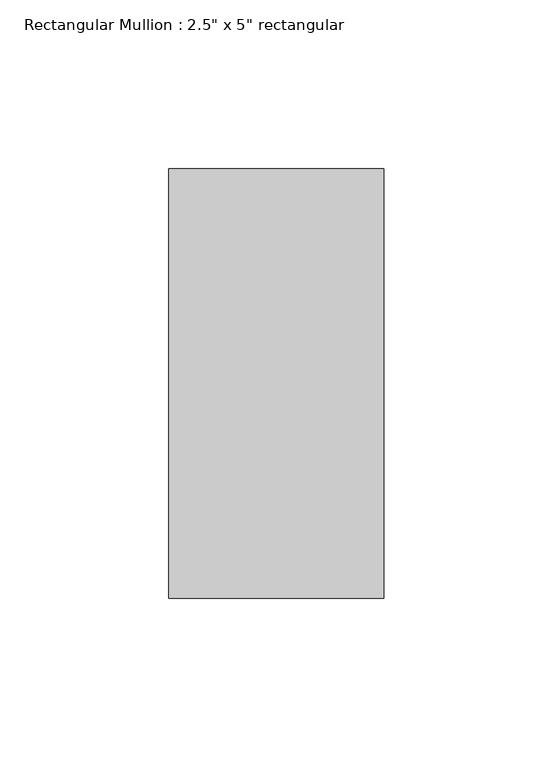
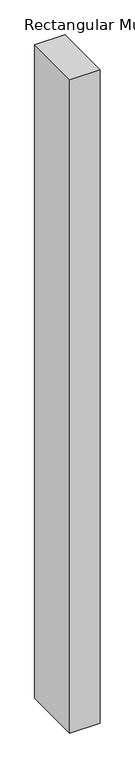
"""IFC4 building model written with IfcOpenShell, lengths in millimetres: member geometry."""

from ifc_helpers import new_model, si_unit, frame, origin, place, context, project, spatial, polyline, outline, extrude, source, transform, mapped, element, save


def member_dbc9f771(model_context):
    return source(origin(), model_context, "Body", "SweptSolid", [
        extrude(outline(polyline([(31.75, 63.5), (31.75, -63.5), (-31.75, -63.5), (-31.75, 63.5), (31.75, 63.5)])), frame((0.0, 0.0, -1446.9814865), z_axis=(0.0, 0.0, 1.0), x_axis=(1.0, 0.0, 0.0)), (0.0, 0.0, 1.0), 1446.9814865),
    ])


if __name__ == "__main__":
    model = new_model("IFC4")
    model_context = context("Model", 3, world=origin())
    ifc_project = project(units=[si_unit("LENGTHUNIT", "METRE", prefix="MILLI")], contexts=[model_context])
    site = spatial("IfcSite", under=ifc_project)
    building = spatial("IfcBuilding", under=site)
    placement = place(None, origin())
    member_shape = member_dbc9f771(model_context)
    element("IfcMember", 1, ObjectType="Rectangular Mullion : 2.5\" x 5\" rectangular", at=placement, inside=building, context=model_context, shape_type="MappedRepresentation", body=[
        mapped(member_shape, transform((0.0, 0.0, 0.0), x_axis=(1.0, 0.0, 0.0), y_axis=(0.0, 1.0, 0.0), z_axis=(0.0, 0.0, 1.0))),
    ])
    save(model, "model.ifc")

# Revit data of these elements
# Type "Rectangular Mullion : 2.5\" x 5\" rectangular"
#   built-in parameter 1007304 = 0.416667 (stored number, unit not read)
#   built-in parameter 1007301 = 0.104167 (stored number, unit not read)
#   built-in parameter 1007300 = 0.104167 (stored number, unit not read)
# Element 1 (IfcMember, "Rectangular Mullion : 2.5\" x 5\" rectangular")
#   Materials on its faces: "Aluminum"
# Materials
#   "Aluminum": class "Metal", colour RGB 247 247 247, transparency 0, Description = "Aluminum 6061", Cost = 0
